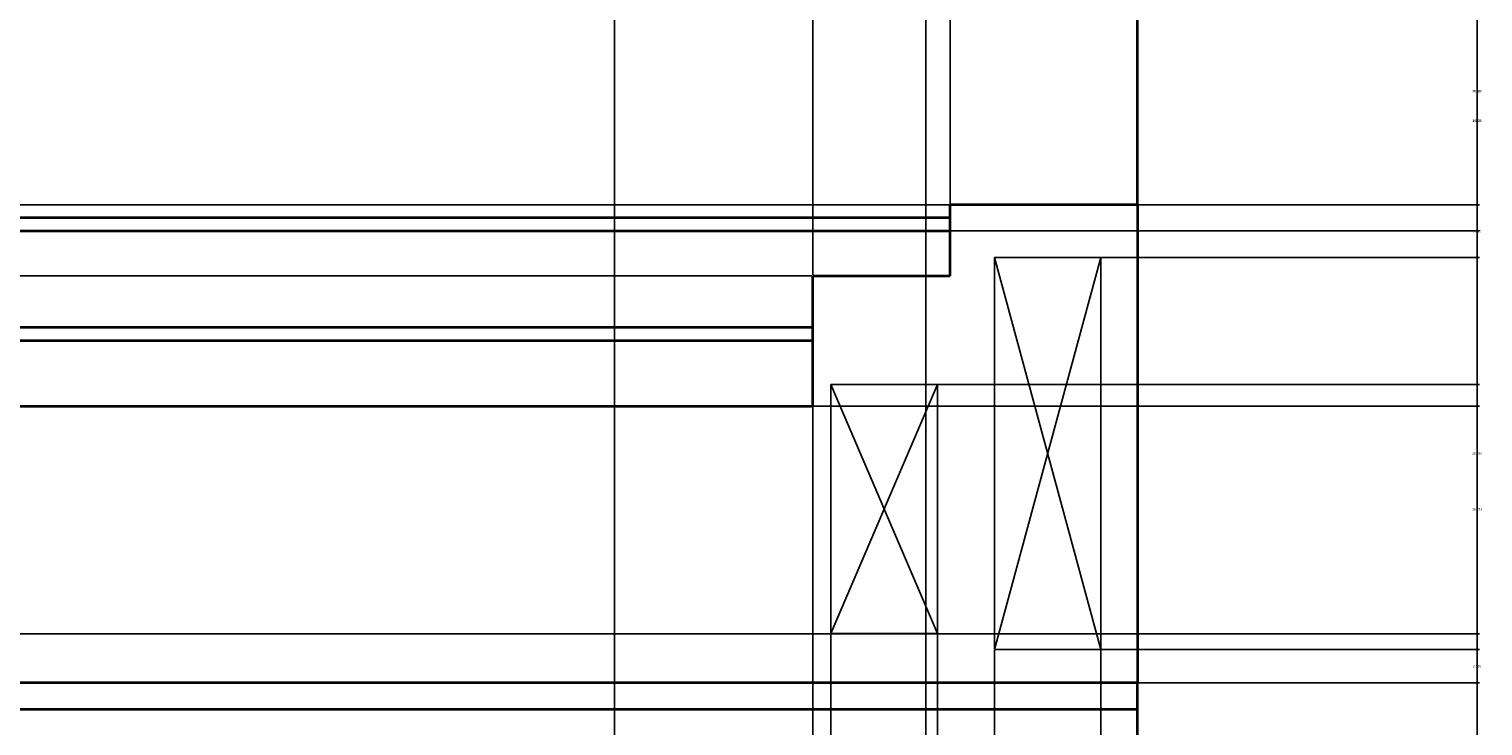
# Model space of a CAD drawing. Units: inches. Extents: x 93 to 565, y 123 to 656.
# Tile 11 of 18: x 456 to 565, y 324 to 377. Entities that reach past the tile are written whole.
import ezdxf

# ---------------------------------------------------------------- set-up
doc = ezdxf.new("R2010")
doc.units = ezdxf.units.IN
doc.header["$MEASUREMENT"] = 0
for name, color, linetype, lineweight in [('A-ANNO-DIMS', 2, 'Continuous', 18), ('A-ELEV', 7, 'Continuous', 35), ('A-GLAZ', 4, 'Continuous', 25)]:
    doc.layers.add(name, color=color, linetype=linetype, lineweight=lineweight)
doc.styles.get("Standard").update_dxf_attribs({"font": 'arial.ttf'})
doc.dimstyles.get("Standard").update_dxf_attribs({"dimtxt": 0.18, "dimasz": 0.18, "dimexe": 0.18, "dimexo": 0.0625, "dimgap": 0.09, "dimtad": 0, "dimtih": 1, "dimtoh": 1, "dimdec": 4, "dimzin": 0, "dimdsep": 46, "dimtxsty": 'Standard', "dimcen": 0.09, "dimadec": 0, "dimazin": 0, "dimtfac": 1, "dimtdec": 4, "dimtofl": 0, "dimtmove": 0, "dimatfit": 3, "dimfxl": 1, "dimtolj": 1, "dimtzin": 0, "dimarcsym": 0})

# ---------------------------------------------------------------- blocks, each defined once
blk = doc.blocks.new('*U8')
for p, q in [((0, 0), (38, 140)), ((38, 0), (0, 140))]:
    blk.add_line(p, q)
blk.add_lwpolyline([(0, 0), (38, 0), (38, 140), (0, 140)], close=True)
blk = doc.blocks.new('*U9')
for p, q in [((0, 0), (38, 89)), ((38, 0), (0, 89))]:
    blk.add_line(p, q)
blk.add_lwpolyline([(0, 0), (38, 0), (38, 89), (0, 89)], close=True)
blk = doc.blocks.new('*D30')
at = {"layer": 'A-ANNO-DIMS', "color": 0, "lineweight": -2, "transparency": 16777216}
for p, q in [((437.19, 594.34), (437.19, 134)), ((539.08, 159.67), (539.08, 134)), ((437.37, 134.18), (487.75, 134.18)), ((538.9, 134.18), (488.52, 134.18))]:
    blk.add_line(p, q, dxfattribs=at)
at = {"layer": 'A-ANNO-DIMS', "color": 0, "transparency": 16777216}
for points in [[(437.37, 134.21), (437.37, 134.15), (437.19, 134.18)], [(538.9, 134.21), (538.9, 134.15), (539.08, 134.18)]]:
    blk.add_solid(points, dxfattribs=at)
at = {"layer": 'Defpoints', "color": 0, "transparency": 16777216}
for p in [(437.19, 594.4), (539.08, 159.73), (539.08, 134.18)]:
    blk.add_point(p, dxfattribs=at)
at = {"layer": 'A-ANNO-DIMS', "color": 0, "transparency": 16777216, "insert": (488.13, 134.18), "char_height": 0.18, "attachment_point": 5}
blk.add_mtext('\\A1;101.9', dxfattribs=at)
blk = doc.blocks.new('*D31')
at = {"layer": 'A-ANNO-DIMS', "color": 0, "lineweight": -2, "transparency": 16777216}
for p, q in [((417.87, 630.4), (564.81, 630.4)), ((564.63, 630.22), (564.63, 395.25)), ((564.63, 159.91), (564.63, 394.89)), ((119.14, 159.73), (564.81, 159.73))]:
    blk.add_line(p, q, dxfattribs=at)
at = {"layer": 'A-ANNO-DIMS', "color": 0, "transparency": 16777216}
for points in [[(564.6, 630.22), (564.66, 630.22), (564.63, 630.4)], [(564.6, 159.91), (564.66, 159.91), (564.63, 159.73)]]:
    blk.add_solid(points, dxfattribs=at)
at = {"layer": 'Defpoints', "color": 0, "transparency": 16777216}
for p in [(417.81, 630.4), (564.63, 630.4), (119.08, 159.73)]:
    blk.add_point(p, dxfattribs=at)
at = {"layer": 'A-ANNO-DIMS', "color": 0, "transparency": 16777216, "insert": (564.63, 395.07), "char_height": 0.18, "attachment_point": 5}
blk.add_mtext('\\A1;470.7', dxfattribs=at)
blk = doc.blocks.new('*D37')
at = {"layer": 'A-ANNO-DIMS', "color": 0, "lineweight": -2, "transparency": 16777216}
for p, q in [((539.14, 327.73), (564.81, 327.73)), ((564.63, 327.55), (564.63, 320.52)), ((564.63, 313.13), (564.63, 320.16)), ((539.14, 312.95), (564.81, 312.95))]:
    blk.add_line(p, q, dxfattribs=at)
at = {"layer": 'A-ANNO-DIMS', "color": 0, "transparency": 16777216}
for points in [[(564.6, 327.55), (564.66, 327.55), (564.63, 327.73)], [(564.6, 313.13), (564.66, 313.13), (564.63, 312.95)]]:
    blk.add_solid(points, dxfattribs=at)
at = {"layer": 'Defpoints', "color": 0, "transparency": 16777216}
for p in [(539.08, 327.73), (564.63, 327.73), (539.08, 312.95)]:
    blk.add_point(p, dxfattribs=at)
at = {"layer": 'A-ANNO-DIMS', "color": 0, "transparency": 16777216, "insert": (564.63, 320.34), "char_height": 0.18, "attachment_point": 5}
blk.add_mtext('\\A1;14.783', dxfattribs=at)
blk = doc.blocks.new('*D67')
at = {"layer": 'A-ANNO-DIMS', "color": 0, "lineweight": -2, "transparency": 16777216}
for p, q in [((331.87, 420.57), (564.81, 420.57)), ((564.63, 420.39), (564.63, 384.75)), ((564.63, 348.75), (564.63, 384.39)), ((331.87, 348.57), (564.81, 348.57))]:
    blk.add_line(p, q, dxfattribs=at)
at = {"layer": 'A-ANNO-DIMS', "color": 0, "transparency": 16777216}
for points in [[(564.6, 420.39), (564.66, 420.39), (564.63, 420.57)], [(564.6, 348.75), (564.66, 348.75), (564.63, 348.57)]]:
    blk.add_solid(points, dxfattribs=at)
at = {"layer": 'Defpoints', "color": 0, "transparency": 16777216}
for p in [(331.81, 420.57), (564.63, 420.57), (331.81, 348.57)]:
    blk.add_point(p, dxfattribs=at)
at = {"layer": 'A-ANNO-DIMS', "color": 0, "transparency": 16777216, "insert": (564.63, 384.57), "char_height": 0.18, "attachment_point": 5}
blk.add_mtext('\\A1;72', dxfattribs=at)
blk = doc.blocks.new('*D71')
at = {"layer": 'A-ANNO-DIMS', "color": 0, "lineweight": -2, "transparency": 16777216}
for p, q in [((428.68, 382.8), (564.81, 382.8)), ((564.63, 382.62), (564.63, 372.46)), ((564.63, 361.93), (564.63, 372.09)), ((437.25, 361.75), (564.81, 361.75))]:
    blk.add_line(p, q, dxfattribs=at)
at = {"layer": 'A-ANNO-DIMS', "color": 0, "transparency": 16777216}
for points in [[(564.6, 382.62), (564.66, 382.62), (564.63, 382.8)], [(564.6, 361.93), (564.66, 361.93), (564.63, 361.75)]]:
    blk.add_solid(points, dxfattribs=at)
at = {"layer": 'Defpoints', "color": 0, "transparency": 16777216}
for p in [(428.62, 382.8), (437.19, 361.75), (564.63, 361.75)]:
    blk.add_point(p, dxfattribs=at)
at = {"layer": 'A-ANNO-DIMS', "color": 0, "transparency": 16777216, "insert": (564.63, 372.27), "char_height": 0.18, "attachment_point": 5}
blk.add_mtext('\\A1;21.05', dxfattribs=at)
blk = doc.blocks.new('*D83')
at = {"layer": 'A-ANNO-DIMS', "color": 0, "lineweight": -2, "transparency": 16777216}
for p, q in [((457.46, 378.34), (564.81, 378.34)), ((564.63, 378.16), (564.63, 370.22)), ((564.63, 361.93), (564.63, 369.86)), ((437.25, 361.75), (564.81, 361.75))]:
    blk.add_line(p, q, dxfattribs=at)
at = {"layer": 'A-ANNO-DIMS', "color": 0, "transparency": 16777216}
for points in [[(564.6, 378.16), (564.66, 378.16), (564.63, 378.34)], [(564.6, 361.93), (564.66, 361.93), (564.63, 361.75)]]:
    blk.add_solid(points, dxfattribs=at)
at = {"layer": 'Defpoints', "color": 0, "transparency": 16777216}
for p in [(457.39, 378.34), (437.19, 361.75), (564.63, 361.75)]:
    blk.add_point(p, dxfattribs=at)
at = {"layer": 'A-ANNO-DIMS', "color": 0, "transparency": 16777216, "insert": (564.63, 370.04), "char_height": 0.18, "attachment_point": 5}
blk.add_mtext('\\A1;16.59', dxfattribs=at)
blk = doc.blocks.new('*D91')
at = {"layer": 'A-ANNO-DIMS', "color": 0, "lineweight": -2, "transparency": 16777216}
for p, q in [((499.73, 599.75), (499.73, 134)), ((437.19, 594.34), (437.19, 134)), ((437.37, 134.18), (468.07, 134.18)), ((499.55, 134.18), (468.85, 134.18))]:
    blk.add_line(p, q, dxfattribs=at)
at = {"layer": 'A-ANNO-DIMS', "color": 0, "transparency": 16777216}
for points in [[(437.37, 134.21), (437.37, 134.15), (437.19, 134.18)], [(499.55, 134.21), (499.55, 134.15), (499.73, 134.18)]]:
    blk.add_solid(points, dxfattribs=at)
at = {"layer": 'Defpoints', "color": 0, "transparency": 16777216}
for p in [(499.73, 599.82), (437.19, 594.4), (499.73, 134.18)]:
    blk.add_point(p, dxfattribs=at)
at = {"layer": 'A-ANNO-DIMS', "color": 0, "transparency": 16777216, "insert": (468.46, 134.18), "char_height": 0.18, "attachment_point": 5}
blk.add_mtext('\\A1;62.54', dxfattribs=at)
blk = doc.blocks.new('*D92')
at = {"layer": 'A-ANNO-DIMS', "color": 0, "lineweight": -2, "transparency": 16777216}
for p, q in [((523.14, 603.14), (523.14, 134)), ((499.73, 599.75), (499.73, 134)), ((499.91, 134.18), (510.97, 134.18)), ((522.96, 134.18), (511.9, 134.18))]:
    blk.add_line(p, q, dxfattribs=at)
at = {"layer": 'A-ANNO-DIMS', "color": 0, "transparency": 16777216}
for points in [[(499.91, 134.21), (499.91, 134.15), (499.73, 134.18)], [(522.96, 134.21), (522.96, 134.15), (523.14, 134.18)]]:
    blk.add_solid(points, dxfattribs=at)
at = {"layer": 'Defpoints', "color": 0, "transparency": 16777216}
for p in [(523.14, 603.2), (499.73, 599.82), (523.14, 134.18)]:
    blk.add_point(p, dxfattribs=at)
at = {"layer": 'A-ANNO-DIMS', "color": 0, "transparency": 16777216, "insert": (511.44, 134.18), "char_height": 0.18, "attachment_point": 5}
blk.add_mtext('\\A1;23.412', dxfattribs=at)
blk = doc.blocks.new('*D93')
at = {"layer": 'A-ANNO-DIMS', "color": 0, "lineweight": -2, "transparency": 16777216}
for p, q in [((523.14, 603.14), (523.14, 134)), ((539.08, 594.34), (539.08, 134)), ((523.32, 134.18), (530.66, 134.18)), ((538.9, 134.18), (531.57, 134.18))]:
    blk.add_line(p, q, dxfattribs=at)
at = {"layer": 'A-ANNO-DIMS', "color": 0, "transparency": 16777216}
for points in [[(523.32, 134.21), (523.32, 134.15), (523.14, 134.18)], [(538.9, 134.21), (538.9, 134.15), (539.08, 134.18)]]:
    blk.add_solid(points, dxfattribs=at)
at = {"layer": 'Defpoints', "color": 0, "transparency": 16777216}
for p in [(523.14, 603.2), (539.08, 594.4), (539.08, 134.18)]:
    blk.add_point(p, dxfattribs=at)
at = {"layer": 'A-ANNO-DIMS', "color": 0, "transparency": 16777216, "insert": (531.11, 134.18), "char_height": 0.18, "attachment_point": 5}
blk.add_mtext('\\A1;15.938', dxfattribs=at)
blk = doc.blocks.new('*D109')
at = {"layer": 'A-ANNO-DIMS', "color": 0, "lineweight": -2, "transparency": 16777216}
for p, q in [((437.19, 594.34), (437.19, 134)), ((539.08, 159.67), (539.08, 134)), ((437.37, 134.18), (487.63, 134.18)), ((538.9, 134.18), (488.64, 134.18))]:
    blk.add_line(p, q, dxfattribs=at)
at = {"layer": 'A-ANNO-DIMS', "color": 0, "transparency": 16777216}
for points in [[(437.37, 134.21), (437.37, 134.15), (437.19, 134.18)], [(538.9, 134.21), (538.9, 134.15), (539.08, 134.18)]]:
    blk.add_solid(points, dxfattribs=at)
at = {"layer": 'Defpoints', "color": 0, "transparency": 16777216}
for p in [(437.19, 594.4), (539.08, 159.73), (539.08, 134.18)]:
    blk.add_point(p, dxfattribs=at)
at = {"layer": 'A-ANNO-DIMS', "color": 0, "transparency": 16777216, "insert": (488.13, 134.18), "char_height": 0.18, "attachment_point": 5}
blk.add_mtext('\\A1;101.891', dxfattribs=at)
blk = doc.blocks.new('*D110')
at = {"layer": 'A-ANNO-DIMS', "color": 0, "lineweight": -2, "transparency": 16777216}
for p, q in [((417.87, 630.4), (564.81, 630.4)), ((564.63, 630.22), (564.63, 395.25)), ((564.63, 159.91), (564.63, 394.89)), ((119.14, 159.73), (564.81, 159.73))]:
    blk.add_line(p, q, dxfattribs=at)
at = {"layer": 'A-ANNO-DIMS', "color": 0, "transparency": 16777216}
for points in [[(564.6, 630.22), (564.66, 630.22), (564.63, 630.4)], [(564.6, 159.91), (564.66, 159.91), (564.63, 159.73)]]:
    blk.add_solid(points, dxfattribs=at)
at = {"layer": 'Defpoints', "color": 0, "transparency": 16777216}
for p in [(417.81, 630.4), (564.63, 630.4), (119.08, 159.73)]:
    blk.add_point(p, dxfattribs=at)
at = {"layer": 'A-ANNO-DIMS', "color": 0, "transparency": 16777216, "insert": (564.63, 395.07), "char_height": 0.18, "attachment_point": 5}
blk.add_mtext('\\A1;470.673', dxfattribs=at)
blk = doc.blocks.new('*D116')
at = {"layer": 'A-ANNO-DIMS', "color": 0, "lineweight": -2, "transparency": 16777216}
for p, q in [((539.14, 327.73), (564.81, 327.73)), ((564.63, 327.55), (564.63, 320.52)), ((564.63, 313.13), (564.63, 320.16)), ((539.14, 312.95), (564.81, 312.95))]:
    blk.add_line(p, q, dxfattribs=at)
at = {"layer": 'A-ANNO-DIMS', "color": 0, "transparency": 16777216}
for points in [[(564.6, 327.55), (564.66, 327.55), (564.63, 327.73)], [(564.6, 313.13), (564.66, 313.13), (564.63, 312.95)]]:
    blk.add_solid(points, dxfattribs=at)
at = {"layer": 'Defpoints', "color": 0, "transparency": 16777216}
for p in [(539.08, 327.73), (564.63, 327.73), (539.08, 312.95)]:
    blk.add_point(p, dxfattribs=at)
at = {"layer": 'A-ANNO-DIMS', "color": 0, "transparency": 16777216, "insert": (564.63, 320.34), "char_height": 0.18, "attachment_point": 5}
blk.add_mtext('\\A1;14.783', dxfattribs=at)
blk = doc.blocks.new('*D146')
at = {"layer": 'A-ANNO-DIMS', "color": 0, "lineweight": -2, "transparency": 16777216}
for p, q in [((331.87, 420.57), (564.81, 420.57)), ((564.63, 420.39), (564.63, 384.75)), ((564.63, 348.75), (564.63, 384.39)), ((331.87, 348.57), (564.81, 348.57))]:
    blk.add_line(p, q, dxfattribs=at)
at = {"layer": 'A-ANNO-DIMS', "color": 0, "transparency": 16777216}
for points in [[(564.6, 420.39), (564.66, 420.39), (564.63, 420.57)], [(564.6, 348.75), (564.66, 348.75), (564.63, 348.57)]]:
    blk.add_solid(points, dxfattribs=at)
at = {"layer": 'Defpoints', "color": 0, "transparency": 16777216}
for p in [(331.81, 420.57), (564.63, 420.57), (331.81, 348.57)]:
    blk.add_point(p, dxfattribs=at)
at = {"layer": 'A-ANNO-DIMS', "color": 0, "transparency": 16777216, "insert": (564.63, 384.57), "char_height": 0.18, "attachment_point": 5}
blk.add_mtext('\\A1;72.000', dxfattribs=at)
blk = doc.blocks.new('*D150')
at = {"layer": 'A-ANNO-DIMS', "color": 0, "lineweight": -2, "transparency": 16777216}
for p, q in [((428.68, 382.8), (564.81, 382.8)), ((564.63, 382.62), (564.63, 372.46)), ((564.63, 361.93), (564.63, 372.09)), ((437.25, 361.75), (564.81, 361.75))]:
    blk.add_line(p, q, dxfattribs=at)
at = {"layer": 'A-ANNO-DIMS', "color": 0, "transparency": 16777216}
for points in [[(564.6, 382.62), (564.66, 382.62), (564.63, 382.8)], [(564.6, 361.93), (564.66, 361.93), (564.63, 361.75)]]:
    blk.add_solid(points, dxfattribs=at)
at = {"layer": 'Defpoints', "color": 0, "transparency": 16777216}
for p in [(428.62, 382.8), (437.19, 361.75), (564.63, 361.75)]:
    blk.add_point(p, dxfattribs=at)
at = {"layer": 'A-ANNO-DIMS', "color": 0, "transparency": 16777216, "insert": (564.63, 372.27), "char_height": 0.18, "attachment_point": 5}
blk.add_mtext('\\A1;21.052', dxfattribs=at)
blk = doc.blocks.new('*D162')
at = {"layer": 'A-ANNO-DIMS', "color": 0, "lineweight": -2, "transparency": 16777216}
for p, q in [((457.46, 378.34), (564.81, 378.34)), ((564.63, 378.16), (564.63, 370.22)), ((564.63, 361.93), (564.63, 369.86)), ((437.25, 361.75), (564.81, 361.75))]:
    blk.add_line(p, q, dxfattribs=at)
at = {"layer": 'A-ANNO-DIMS', "color": 0, "transparency": 16777216}
for points in [[(564.6, 378.16), (564.66, 378.16), (564.63, 378.34)], [(564.6, 361.93), (564.66, 361.93), (564.63, 361.75)]]:
    blk.add_solid(points, dxfattribs=at)
at = {"layer": 'Defpoints', "color": 0, "transparency": 16777216}
for p in [(457.39, 378.34), (437.19, 361.75), (564.63, 361.75)]:
    blk.add_point(p, dxfattribs=at)
at = {"layer": 'A-ANNO-DIMS', "color": 0, "transparency": 16777216, "insert": (564.63, 370.04), "char_height": 0.18, "attachment_point": 5}
blk.add_mtext('\\A1;16.590', dxfattribs=at)
blk = doc.blocks.new('*D170')
at = {"layer": 'A-ANNO-DIMS', "color": 0, "lineweight": -2, "transparency": 16777216}
for p, q in [((499.73, 599.75), (499.73, 134)), ((437.19, 594.34), (437.19, 134)), ((437.37, 134.18), (468.01, 134.18)), ((499.55, 134.18), (468.91, 134.18))]:
    blk.add_line(p, q, dxfattribs=at)
at = {"layer": 'A-ANNO-DIMS', "color": 0, "transparency": 16777216}
for points in [[(437.37, 134.21), (437.37, 134.15), (437.19, 134.18)], [(499.55, 134.21), (499.55, 134.15), (499.73, 134.18)]]:
    blk.add_solid(points, dxfattribs=at)
at = {"layer": 'Defpoints', "color": 0, "transparency": 16777216}
for p in [(499.73, 599.82), (437.19, 594.4), (499.73, 134.18)]:
    blk.add_point(p, dxfattribs=at)
at = {"layer": 'A-ANNO-DIMS', "color": 0, "transparency": 16777216, "insert": (468.46, 134.18), "char_height": 0.18, "attachment_point": 5}
blk.add_mtext('\\A1;62.541', dxfattribs=at)
blk = doc.blocks.new('*D171')
at = {"layer": 'A-ANNO-DIMS', "color": 0, "lineweight": -2, "transparency": 16777216}
for p, q in [((523.14, 603.14), (523.14, 134)), ((499.73, 599.75), (499.73, 134)), ((499.91, 134.18), (510.97, 134.18)), ((522.96, 134.18), (511.9, 134.18))]:
    blk.add_line(p, q, dxfattribs=at)
at = {"layer": 'A-ANNO-DIMS', "color": 0, "transparency": 16777216}
for points in [[(499.91, 134.21), (499.91, 134.15), (499.73, 134.18)], [(522.96, 134.21), (522.96, 134.15), (523.14, 134.18)]]:
    blk.add_solid(points, dxfattribs=at)
at = {"layer": 'Defpoints', "color": 0, "transparency": 16777216}
for p in [(523.14, 603.2), (499.73, 599.82), (523.14, 134.18)]:
    blk.add_point(p, dxfattribs=at)
at = {"layer": 'A-ANNO-DIMS', "color": 0, "transparency": 16777216, "insert": (511.44, 134.18), "char_height": 0.18, "attachment_point": 5}
blk.add_mtext('\\A1;23.412', dxfattribs=at)
blk = doc.blocks.new('*D172')
at = {"layer": 'A-ANNO-DIMS', "color": 0, "lineweight": -2, "transparency": 16777216}
for p, q in [((523.14, 603.14), (523.14, 134)), ((539.08, 594.34), (539.08, 134)), ((523.32, 134.18), (530.66, 134.18)), ((538.9, 134.18), (531.57, 134.18))]:
    blk.add_line(p, q, dxfattribs=at)
at = {"layer": 'A-ANNO-DIMS', "color": 0, "transparency": 16777216}
for points in [[(523.32, 134.21), (523.32, 134.15), (523.14, 134.18)], [(538.9, 134.21), (538.9, 134.15), (539.08, 134.18)]]:
    blk.add_solid(points, dxfattribs=at)
at = {"layer": 'Defpoints', "color": 0, "transparency": 16777216}
for p in [(523.14, 603.2), (539.08, 594.4), (539.08, 134.18)]:
    blk.add_point(p, dxfattribs=at)
at = {"layer": 'A-ANNO-DIMS', "color": 0, "transparency": 16777216, "insert": (531.11, 134.18), "char_height": 0.18, "attachment_point": 5}
blk.add_mtext('\\A1;15.938', dxfattribs=at)
blk = doc.blocks.new('*D180')
at = {"layer": 'A-ANNO-DIMS', "color": 0, "lineweight": -2, "transparency": 16777216}
for p, q in [((514.64, 348.49), (514.64, 134)), ((516.01, 331.37), (516.01, 134)), ((514.82, 134.18), (514.94, 134.18)), ((515.83, 134.18), (515.71, 134.18))]:
    blk.add_line(p, q, dxfattribs=at)
at = {"layer": 'A-ANNO-DIMS', "color": 0, "transparency": 16777216}
for points in [[(514.82, 134.21), (514.82, 134.15), (514.64, 134.18)], [(515.83, 134.21), (515.83, 134.15), (516.01, 134.18)]]:
    blk.add_solid(points, dxfattribs=at)
at = {"layer": 'Defpoints', "color": 0, "transparency": 16777216}
for p in [(514.64, 348.55), (516.01, 331.43), (516.01, 134.18)]:
    blk.add_point(p, dxfattribs=at)
at = {"layer": 'A-ANNO-DIMS', "color": 0, "transparency": 16777216, "insert": (515.33, 134.18), "char_height": 0.18, "attachment_point": 5}
blk.add_mtext('\\A1;1.367', dxfattribs=at)
blk = doc.blocks.new('*D181')
at = {"layer": 'A-ANNO-DIMS', "color": 0, "lineweight": -2, "transparency": 16777216}
for p, q in [((516.01, 331.37), (516.01, 134)), ((524.02, 331.37), (524.02, 134)), ((516.19, 134.18), (519.62, 134.18)), ((523.84, 134.18), (520.41, 134.18))]:
    blk.add_line(p, q, dxfattribs=at)
at = {"layer": 'A-ANNO-DIMS', "color": 0, "transparency": 16777216}
for points in [[(516.19, 134.21), (516.19, 134.15), (516.01, 134.18)], [(523.84, 134.21), (523.84, 134.15), (524.02, 134.18)]]:
    blk.add_solid(points, dxfattribs=at)
at = {"layer": 'Defpoints', "color": 0, "transparency": 16777216}
for p in [(516.01, 331.43), (524.02, 331.43), (524.02, 134.18)]:
    blk.add_point(p, dxfattribs=at)
at = {"layer": 'A-ANNO-DIMS', "color": 0, "transparency": 16777216, "insert": (520.01, 134.18), "char_height": 0.18, "attachment_point": 5}
blk.add_mtext('\\A1;8.007', dxfattribs=at)
blk = doc.blocks.new('*D182')
at = {"layer": 'A-ANNO-DIMS', "color": 0, "lineweight": -2, "transparency": 16777216}
for p, q in [((524.02, 331.37), (524.02, 134)), ((528.31, 330.19), (528.31, 134)), ((524.2, 134.18), (525.77, 134.18)), ((528.13, 134.18), (526.56, 134.18))]:
    blk.add_line(p, q, dxfattribs=at)
at = {"layer": 'A-ANNO-DIMS', "color": 0, "transparency": 16777216}
for points in [[(524.2, 134.21), (524.2, 134.15), (524.02, 134.18)], [(528.13, 134.21), (528.13, 134.15), (528.31, 134.18)]]:
    blk.add_solid(points, dxfattribs=at)
at = {"layer": 'Defpoints', "color": 0, "transparency": 16777216}
for p in [(524.02, 331.43), (528.31, 330.25), (528.31, 134.18)]:
    blk.add_point(p, dxfattribs=at)
at = {"layer": 'A-ANNO-DIMS', "color": 0, "transparency": 16777216, "insert": (526.17, 134.18), "char_height": 0.18, "attachment_point": 5}
blk.add_mtext('\\A1;4.297', dxfattribs=at)
blk = doc.blocks.new('*D183')
at = {"layer": 'A-ANNO-DIMS', "color": 0, "lineweight": -2, "transparency": 16777216}
for p, q in [((528.31, 330.19), (528.31, 134)), ((536.32, 330.19), (536.32, 134)), ((528.49, 134.18), (531.92, 134.18)), ((536.14, 134.18), (532.71, 134.18))]:
    blk.add_line(p, q, dxfattribs=at)
at = {"layer": 'A-ANNO-DIMS', "color": 0, "transparency": 16777216}
for points in [[(528.49, 134.21), (528.49, 134.15), (528.31, 134.18)], [(536.14, 134.21), (536.14, 134.15), (536.32, 134.18)]]:
    blk.add_solid(points, dxfattribs=at)
at = {"layer": 'Defpoints', "color": 0, "transparency": 16777216}
for p in [(528.31, 330.25), (536.32, 330.25), (536.32, 134.18)]:
    blk.add_point(p, dxfattribs=at)
at = {"layer": 'A-ANNO-DIMS', "color": 0, "transparency": 16777216, "insert": (532.32, 134.18), "char_height": 0.18, "attachment_point": 5}
blk.add_mtext('\\A1;8.007', dxfattribs=at)
blk = doc.blocks.new('*D184')
at = {"layer": 'A-ANNO-DIMS', "color": 0, "lineweight": -2, "transparency": 16777216}
for p, q in [((536.32, 330.19), (536.32, 134)), ((539.08, 327.67), (539.08, 134)), ((536.5, 134.18), (537.31, 134.18)), ((538.9, 134.18), (538.1, 134.18))]:
    blk.add_line(p, q, dxfattribs=at)
at = {"layer": 'A-ANNO-DIMS', "color": 0, "transparency": 16777216}
for points in [[(536.5, 134.21), (536.5, 134.15), (536.32, 134.18)], [(538.9, 134.21), (538.9, 134.15), (539.08, 134.18)]]:
    blk.add_solid(points, dxfattribs=at)
at = {"layer": 'Defpoints', "color": 0, "transparency": 16777216}
for p in [(536.32, 330.25), (539.08, 327.73), (539.08, 134.18)]:
    blk.add_point(p, dxfattribs=at)
at = {"layer": 'A-ANNO-DIMS', "color": 0, "transparency": 16777216, "insert": (537.7, 134.18), "char_height": 0.18, "attachment_point": 5}
blk.add_mtext('\\A1;2.758', dxfattribs=at)
blk = doc.blocks.new('*D185')
at = {"layer": 'A-ANNO-DIMS', "color": 0, "lineweight": -2, "transparency": 16777216}
for p, q in [((514.64, 358.44), (514.64, 656.13)), ((514.82, 655.95), (519.36, 655.95)), ((524.81, 655.95), (520.27, 655.95)), ((524.99, 363.79), (524.99, 656.13))]:
    blk.add_line(p, q, dxfattribs=at)
at = {"layer": 'A-ANNO-DIMS', "color": 0, "transparency": 16777216}
for points in [[(514.82, 655.98), (514.82, 655.92), (514.64, 655.95)], [(524.81, 655.98), (524.81, 655.92), (524.99, 655.95)]]:
    blk.add_solid(points, dxfattribs=at)
at = {"layer": 'Defpoints', "color": 0, "transparency": 16777216}
for p in [(524.99, 655.95), (524.99, 363.73), (514.64, 358.37)]:
    blk.add_point(p, dxfattribs=at)
at = {"layer": 'A-ANNO-DIMS', "color": 0, "transparency": 16777216, "insert": (519.81, 655.95), "char_height": 0.18, "attachment_point": 5}
blk.add_mtext('\\A1;10.344', dxfattribs=at)
blk = doc.blocks.new('*D186')
at = {"layer": 'A-ANNO-DIMS', "color": 0, "lineweight": -2, "transparency": 16777216}
for p, q in [((524.99, 363.79), (524.99, 656.13)), ((525.17, 655.95), (531.58, 655.95)), ((538.9, 655.95), (532.49, 655.95)), ((539.08, 363.79), (539.08, 656.13))]:
    blk.add_line(p, q, dxfattribs=at)
at = {"layer": 'A-ANNO-DIMS', "color": 0, "transparency": 16777216}
for points in [[(525.17, 655.98), (525.17, 655.92), (524.99, 655.95)], [(538.9, 655.98), (538.9, 655.92), (539.08, 655.95)]]:
    blk.add_solid(points, dxfattribs=at)
at = {"layer": 'Defpoints', "color": 0, "transparency": 16777216}
for p in [(539.08, 655.95), (524.99, 363.73), (539.08, 363.73)]:
    blk.add_point(p, dxfattribs=at)
at = {"layer": 'A-ANNO-DIMS', "color": 0, "transparency": 16777216, "insert": (532.03, 655.95), "char_height": 0.18, "attachment_point": 5}
blk.add_mtext('\\A1;14.093', dxfattribs=at)
blk = doc.blocks.new('*D187')
at = {"layer": 'A-ANNO-DIMS', "color": 0, "lineweight": -2, "transparency": 16777216}
for p, q in [((536.38, 330.25), (564.81, 330.25)), ((564.63, 330.07), (564.63, 329.17)), ((564.63, 327.91), (564.63, 328.81)), ((539.14, 327.73), (564.81, 327.73))]:
    blk.add_line(p, q, dxfattribs=at)
at = {"layer": 'A-ANNO-DIMS', "color": 0, "transparency": 16777216}
for points in [[(564.6, 330.07), (564.66, 330.07), (564.63, 330.25)], [(564.6, 327.91), (564.66, 327.91), (564.63, 327.73)]]:
    blk.add_solid(points, dxfattribs=at)
at = {"layer": 'Defpoints', "color": 0, "transparency": 16777216}
for p in [(536.32, 330.25), (564.63, 330.25), (539.08, 327.73)]:
    blk.add_point(p, dxfattribs=at)
at = {"layer": 'A-ANNO-DIMS', "color": 0, "transparency": 16777216, "insert": (564.63, 328.99), "char_height": 0.18, "attachment_point": 5}
blk.add_mtext('\\A1;2.516', dxfattribs=at)
blk = doc.blocks.new('*D188')
at = {"layer": 'A-ANNO-DIMS', "color": 0, "lineweight": -2, "transparency": 16777216}
for p, q in [((536.38, 359.75), (564.81, 359.75)), ((564.63, 359.57), (564.63, 345.18)), ((564.63, 330.43), (564.63, 344.82)), ((536.38, 330.25), (564.81, 330.25))]:
    blk.add_line(p, q, dxfattribs=at)
at = {"layer": 'A-ANNO-DIMS', "color": 0, "transparency": 16777216}
for points in [[(564.6, 359.57), (564.66, 359.57), (564.63, 359.75)], [(564.6, 330.43), (564.66, 330.43), (564.63, 330.25)]]:
    blk.add_solid(points, dxfattribs=at)
at = {"layer": 'Defpoints', "color": 0, "transparency": 16777216}
for p in [(536.32, 359.75), (564.63, 359.75), (536.32, 330.25)]:
    blk.add_point(p, dxfattribs=at)
at = {"layer": 'A-ANNO-DIMS', "color": 0, "transparency": 16777216, "insert": (564.63, 345), "char_height": 0.18, "attachment_point": 5}
blk.add_mtext('\\A1;29.500', dxfattribs=at)
blk = doc.blocks.new('*D189')
at = {"layer": 'A-ANNO-DIMS', "color": 0, "lineweight": -2, "transparency": 16777216}
for p, q in [((539.14, 363.73), (564.81, 363.73)), ((564.63, 363.55), (564.63, 361.92)), ((564.63, 359.93), (564.63, 361.56)), ((536.38, 359.75), (564.81, 359.75))]:
    blk.add_line(p, q, dxfattribs=at)
at = {"layer": 'A-ANNO-DIMS', "color": 0, "transparency": 16777216}
for points in [[(564.6, 363.55), (564.66, 363.55), (564.63, 363.73)], [(564.6, 359.93), (564.66, 359.93), (564.63, 359.75)]]:
    blk.add_solid(points, dxfattribs=at)
at = {"layer": 'Defpoints', "color": 0, "transparency": 16777216}
for p in [(539.08, 363.73), (564.63, 363.73), (536.32, 359.75)]:
    blk.add_point(p, dxfattribs=at)
at = {"layer": 'A-ANNO-DIMS', "color": 0, "transparency": 16777216, "insert": (564.63, 361.74), "char_height": 0.18, "attachment_point": 5}
blk.add_mtext('\\A1;3.985', dxfattribs=at)
blk = doc.blocks.new('*D190')
at = {"layer": 'A-ANNO-DIMS', "color": 0, "lineweight": -2, "transparency": 16777216}
for p, q in [((514.58, 348.55), (93.35, 348.55)), ((93.53, 348.37), (93.53, 338.33)), ((93.53, 327.91), (93.53, 337.96)), ((539.02, 327.73), (93.35, 327.73))]:
    blk.add_line(p, q, dxfattribs=at)
at = {"layer": 'A-ANNO-DIMS', "color": 0, "transparency": 16777216}
for points in [[(93.5, 348.37), (93.56, 348.37), (93.53, 348.55)], [(93.5, 327.91), (93.56, 327.91), (93.53, 327.73)]]:
    blk.add_solid(points, dxfattribs=at)
at = {"layer": 'Defpoints', "color": 0, "transparency": 16777216}
for p in [(93.53, 348.55), (514.64, 348.55), (539.08, 327.73)]:
    blk.add_point(p, dxfattribs=at)
at = {"layer": 'A-ANNO-DIMS', "color": 0, "transparency": 16777216, "insert": (93.53, 338.14), "char_height": 0.18, "attachment_point": 5}
blk.add_mtext('\\A1;20.822', dxfattribs=at)
blk = doc.blocks.new('*D191')
at = {"layer": 'A-ANNO-DIMS', "color": 0, "lineweight": -2, "transparency": 16777216}
for p, q in [((514.58, 353.47), (93.35, 353.47)), ((93.53, 353.29), (93.53, 351.2)), ((93.53, 348.73), (93.53, 350.83)), ((514.58, 348.55), (93.35, 348.55))]:
    blk.add_line(p, q, dxfattribs=at)
at = {"layer": 'A-ANNO-DIMS', "color": 0, "transparency": 16777216}
for points in [[(93.5, 353.29), (93.56, 353.29), (93.53, 353.47)], [(93.5, 348.73), (93.56, 348.73), (93.53, 348.55)]]:
    blk.add_solid(points, dxfattribs=at)
at = {"layer": 'Defpoints', "color": 0, "transparency": 16777216}
for p in [(93.53, 353.47), (514.64, 353.47), (514.64, 348.55)]:
    blk.add_point(p, dxfattribs=at)
at = {"layer": 'A-ANNO-DIMS', "color": 0, "transparency": 16777216, "insert": (93.53, 351.01), "char_height": 0.18, "attachment_point": 5}
blk.add_mtext('\\A1;4.918', dxfattribs=at)
blk = doc.blocks.new('*D192')
at = {"layer": 'A-ANNO-DIMS', "color": 0, "lineweight": -2, "transparency": 16777216}
for p, q in [((514.58, 354.47), (93.35, 354.47)), ((514.58, 353.47), (93.35, 353.47)), ((93.53, 354.29), (93.53, 354.15)), ((93.53, 353.65), (93.53, 353.79))]:
    blk.add_line(p, q, dxfattribs=at)
at = {"layer": 'A-ANNO-DIMS', "color": 0, "transparency": 16777216}
for points in [[(93.5, 354.29), (93.56, 354.29), (93.53, 354.47)], [(93.5, 353.65), (93.56, 353.65), (93.53, 353.47)]]:
    blk.add_solid(points, dxfattribs=at)
at = {"layer": 'Defpoints', "color": 0, "transparency": 16777216}
for p in [(93.53, 354.47), (514.64, 354.47), (514.64, 353.47)]:
    blk.add_point(p, dxfattribs=at)
at = {"layer": 'A-ANNO-DIMS', "color": 0, "transparency": 16777216, "insert": (93.53, 353.97), "char_height": 0.18, "attachment_point": 5}
blk.add_mtext('\\A1;1.000', dxfattribs=at)
blk = doc.blocks.new('*D193')
at = {"layer": 'A-ANNO-DIMS', "color": 0, "lineweight": -2, "transparency": 16777216}
for p, q in [((514.58, 358.37), (93.35, 358.37)), ((93.53, 358.19), (93.53, 356.61)), ((93.53, 354.65), (93.53, 356.24)), ((514.58, 354.47), (93.35, 354.47))]:
    blk.add_line(p, q, dxfattribs=at)
at = {"layer": 'A-ANNO-DIMS', "color": 0, "transparency": 16777216}
for points in [[(93.5, 358.19), (93.56, 358.19), (93.53, 358.37)], [(93.5, 354.65), (93.56, 354.65), (93.53, 354.47)]]:
    blk.add_solid(points, dxfattribs=at)
at = {"layer": 'Defpoints', "color": 0, "transparency": 16777216}
for p in [(93.53, 358.37), (514.64, 358.37), (514.64, 354.47)]:
    blk.add_point(p, dxfattribs=at)
at = {"layer": 'A-ANNO-DIMS', "color": 0, "transparency": 16777216, "insert": (93.53, 356.42), "char_height": 0.18, "attachment_point": 5}
blk.add_mtext('\\A1;3.901', dxfattribs=at)
blk = doc.blocks.new('*D194')
at = {"layer": 'A-ANNO-DIMS', "color": 0, "lineweight": -2, "transparency": 16777216}
for p, q in [((524.92, 361.75), (93.35, 361.75)), ((93.53, 361.57), (93.53, 360.24)), ((93.53, 358.55), (93.53, 359.88)), ((514.58, 358.37), (93.35, 358.37))]:
    blk.add_line(p, q, dxfattribs=at)
at = {"layer": 'A-ANNO-DIMS', "color": 0, "transparency": 16777216}
for points in [[(93.5, 361.57), (93.56, 361.57), (93.53, 361.75)], [(93.5, 358.55), (93.56, 358.55), (93.53, 358.37)]]:
    blk.add_solid(points, dxfattribs=at)
at = {"layer": 'Defpoints', "color": 0, "transparency": 16777216}
for p in [(93.53, 361.75), (524.99, 361.75), (514.64, 358.37)]:
    blk.add_point(p, dxfattribs=at)
at = {"layer": 'A-ANNO-DIMS', "color": 0, "transparency": 16777216, "insert": (93.53, 360.06), "char_height": 0.18, "attachment_point": 5}
blk.add_mtext('\\A1;3.374', dxfattribs=at)
blk = doc.blocks.new('*D195')
at = {"layer": 'A-ANNO-DIMS', "color": 0, "lineweight": -2, "transparency": 16777216}
for p, q in [((524.92, 362.75), (93.35, 362.75)), ((93.53, 362.57), (93.53, 362.43)), ((524.92, 361.75), (93.35, 361.75)), ((93.53, 361.93), (93.53, 362.07))]:
    blk.add_line(p, q, dxfattribs=at)
at = {"layer": 'A-ANNO-DIMS', "color": 0, "transparency": 16777216}
for points in [[(93.5, 362.57), (93.56, 362.57), (93.53, 362.75)], [(93.5, 361.93), (93.56, 361.93), (93.53, 361.75)]]:
    blk.add_solid(points, dxfattribs=at)
at = {"layer": 'Defpoints', "color": 0, "transparency": 16777216}
for p in [(93.53, 362.75), (524.99, 362.75), (524.99, 361.75)]:
    blk.add_point(p, dxfattribs=at)
at = {"layer": 'A-ANNO-DIMS', "color": 0, "transparency": 16777216, "insert": (93.53, 362.25), "char_height": 0.18, "attachment_point": 5}
blk.add_mtext('\\A1;1.000', dxfattribs=at)
blk = doc.blocks.new('*D196')
at = {"layer": 'A-ANNO-DIMS', "color": 0, "lineweight": -2, "transparency": 16777216}
for p, q in [((524.92, 363.73), (93.35, 363.73)), ((93.53, 363.55), (93.53, 363.42)), ((524.92, 362.75), (93.35, 362.75)), ((93.53, 362.93), (93.53, 363.06))]:
    blk.add_line(p, q, dxfattribs=at)
at = {"layer": 'A-ANNO-DIMS', "color": 0, "transparency": 16777216}
for points in [[(93.5, 363.55), (93.56, 363.55), (93.53, 363.73)], [(93.5, 362.93), (93.56, 362.93), (93.53, 362.75)]]:
    blk.add_solid(points, dxfattribs=at)
at = {"layer": 'Defpoints', "color": 0, "transparency": 16777216}
for p in [(93.53, 363.73), (524.99, 363.73), (524.99, 362.75)]:
    blk.add_point(p, dxfattribs=at)
at = {"layer": 'A-ANNO-DIMS', "color": 0, "transparency": 16777216, "insert": (93.53, 363.24), "char_height": 0.18, "attachment_point": 5}
blk.add_mtext('\\A1;0.985', dxfattribs=at)
blk = doc.blocks.new('*D197')
at = {"layer": 'A-ANNO-DIMS', "color": 0, "lineweight": -2, "transparency": 16777216}
for p, q in [((516.07, 350.19), (564.81, 350.19)), ((564.63, 350.01), (564.63, 340.99)), ((564.63, 331.61), (564.63, 340.63)), ((516.07, 331.43), (564.81, 331.43))]:
    blk.add_line(p, q, dxfattribs=at)
at = {"layer": 'A-ANNO-DIMS', "color": 0, "transparency": 16777216}
for points in [[(564.6, 350.01), (564.66, 350.01), (564.63, 350.19)], [(564.6, 331.61), (564.66, 331.61), (564.63, 331.43)]]:
    blk.add_solid(points, dxfattribs=at)
at = {"layer": 'Defpoints', "color": 0, "transparency": 16777216}
for p in [(516.01, 350.19), (564.63, 350.19), (516.01, 331.43)]:
    blk.add_point(p, dxfattribs=at)
at = {"layer": 'A-ANNO-DIMS', "color": 0, "transparency": 16777216, "insert": (564.63, 340.81), "char_height": 0.18, "attachment_point": 5}
blk.add_mtext('\\A1;18.753', dxfattribs=at)
blk = doc.blocks.new('*D198')
at = {"layer": 'A-ANNO-DIMS', "color": 0, "lineweight": -2, "transparency": 16777216}
for p, q in [((515.95, 331.43), (93.35, 331.43)), ((93.53, 331.25), (93.53, 329.76)), ((93.53, 327.91), (93.53, 329.4)), ((539.02, 327.73), (93.35, 327.73))]:
    blk.add_line(p, q, dxfattribs=at)
at = {"layer": 'A-ANNO-DIMS', "color": 0, "transparency": 16777216}
for points in [[(93.5, 331.25), (93.56, 331.25), (93.53, 331.43)], [(93.5, 327.91), (93.56, 327.91), (93.53, 327.73)]]:
    blk.add_solid(points, dxfattribs=at)
at = {"layer": 'Defpoints', "color": 0, "transparency": 16777216}
for p in [(93.53, 331.43), (516.01, 331.43), (539.08, 327.73)]:
    blk.add_point(p, dxfattribs=at)
at = {"layer": 'A-ANNO-DIMS', "color": 0, "transparency": 16777216, "insert": (93.53, 329.58), "char_height": 0.18, "attachment_point": 5}
blk.add_mtext('\\A1;3.701', dxfattribs=at)

msp = doc.modelspace()

# ---------------------------------------------------------------- linework, layer by layer
at = {"layer": 'A-ELEV'}
for p, q in [((539.0794, 363.7323), (539.0794, 594.4048)), ((524.9864, 358.3735), (524.9864, 363.7323)), ((524.9864, 363.7323), (539.0794, 363.7323)), ((539.0794, 363.7323), (539.0794, 327.7323)), ((524.9864, 362.7477), (295.6874, 362.7477)), ((524.9864, 361.7477), (295.6874, 361.7477)), ((514.6424, 348.5546), (514.6424, 358.3735)), ((514.6424, 358.3735), (524.9864, 358.3735)), ((514.6424, 354.4729), (295.6874, 354.4729)), ((514.6424, 353.4729), (295.6874, 353.4729)), ((295.6874, 348.5546), (514.6424, 348.5546)), ((539.0794, 327.7323), (295.6874, 327.7323)), ((539.0794, 183.7323), (539.0794, 327.7323)), ((539.0794, 325.7323), (295.6874, 325.7323))]:
    msp.add_line(p, q, dxfattribs=at)

# ---------------------------------------------------------------- block references
at = {"layer": 'A-GLAZ', "xscale": 0.2107133031769033, "yscale": 0.2107133031769033, "zscale": 0.2107133031769033}
for name, p in [('*U8', (528.3144, 330.2478)), ('*U9', (516.0099, 331.4335))]:
    msp.add_blockref(name, p, dxfattribs=at)

# ---------------------------------------------------------------- dimensions: what is measured, and where the dimension line sits
at = {"layer": 'A-ANNO-DIMS'}
for base, p1, p2, override, picture, middle in [((524.9864, 655.9548), (514.6424, 358.3735), (524.9864, 363.7323), {"dimdec": 3, "dimlfac": 1, "dimrnd": 0, "dimzin": 0, "dimdsep": 46, "dimlunit": 2}, '*D185', (519.8144, 655.9548)), ((539.0794, 655.9548), (524.9864, 363.7323), (539.0794, 363.7323), {"dimdec": 3, "dimlfac": 1, "dimrnd": 0, "dimzin": 0, "dimdsep": 46, "dimlunit": 2}, '*D186', (532.0329, 655.9548)), ((523.1415, 134.1823), (499.7291, 599.8171), (523.1415, 603.1979), {"dimdec": 3, "dimlfac": 1, "dimrnd": 0, "dimzin": 0, "dimdsep": 46, "dimlunit": 2}, '*D92', (511.4353, 134.1823)), ((523.1415, 134.1823), (499.7291, 599.8171), (523.1415, 603.1979), {"dimdec": 3, "dimlfac": 1, "dimrnd": 0, "dimzin": 0, "dimdsep": 46, "dimlunit": 2}, '*D171', (511.4353, 134.1823)), ((539.0794, 134.1823), (523.1415, 603.1979), (539.0794, 594.4048), {"dimdec": 3, "dimlfac": 1, "dimrnd": 0, "dimzin": 0, "dimdsep": 46, "dimlunit": 2}, '*D93', (531.1104, 134.1823)), ((539.0794, 134.1823), (523.1415, 603.1979), (539.0794, 594.4048), {"dimdec": 3, "dimlfac": 1, "dimrnd": 0, "dimzin": 0, "dimdsep": 46, "dimlunit": 2}, '*D172', (531.1104, 134.1823)), ((499.7291, 134.1823), (437.1885, 594.4048), (499.7291, 599.8171), {"dimdec": 2, "dimlfac": 1, "dimrnd": 0, "dimzin": 0, "dimdsep": 46, "dimlunit": 2}, '*D91', (468.4588, 134.1823)), ((499.7291, 134.1823), (437.1885, 594.4048), (499.7291, 599.8171), {"dimdec": 3, "dimlfac": 1, "dimrnd": 0, "dimzin": 0, "dimdsep": 46, "dimlunit": 2}, '*D170', (468.4588, 134.1823)), ((539.0794, 134.1823), (437.1885, 594.4048), (539.0794, 159.7323), {"dimdec": 1, "dimlfac": 1, "dimrnd": 0, "dimzin": 0, "dimdsep": 46, "dimlunit": 2}, '*D30', (488.1339, 134.1823)), ((539.0794, 134.1823), (437.1885, 594.4048), (539.0794, 159.7323), {"dimdec": 3, "dimlfac": 1, "dimrnd": 0, "dimzin": 0, "dimdsep": 46, "dimlunit": 2}, '*D109', (488.1339, 134.1823)), ((516.00989, 134.18225), (514.64241, 348.5546), (516.00989, 331.43349), {"dimdec": 3, "dimlfac": 1, "dimrnd": 0, "dimzin": 0, "dimdsep": 46, "dimlunit": 2}, '*D180', (515.32615, 134.18225)), ((524.017, 134.1823), (516.0099, 331.4335), (524.017, 331.4335), {"dimdec": 3, "dimlfac": 1, "dimrnd": 0, "dimzin": 0, "dimdsep": 46, "dimlunit": 2}, '*D181', (520.0134, 134.1823)), ((528.3144, 134.1823), (524.017, 331.4335), (528.3144, 330.2478), {"dimdec": 3, "dimlfac": 1, "dimrnd": 0, "dimzin": 0, "dimdsep": 46, "dimlunit": 2}, '*D182', (526.1657, 134.1823)), ((536.3215, 134.1823), (528.3144, 330.2478), (536.3215, 330.2478), {"dimdec": 3, "dimlfac": 1, "dimrnd": 0, "dimzin": 0, "dimdsep": 46, "dimlunit": 2}, '*D183', (532.318, 134.1823)), ((539.0794, 134.1823), (536.3215, 330.2478), (539.0794, 327.7323), {"dimdec": 3, "dimlfac": 1, "dimrnd": 0, "dimzin": 0, "dimdsep": 46, "dimlunit": 2}, '*D184', (537.7004, 134.1823))]:
    dim = msp.add_linear_dim(base=base, p1=p1, p2=p2, dimstyle='Standard', override=override, dxfattribs=at)
    dim.commit()
    dim.dimension.update_dxf_attribs({"geometry": picture, "text_midpoint": middle})
for base, p1, p2, override, picture, middle in [((564.6294, 630.4048), (119.0794, 159.7323), (417.8097, 630.4048), {"dimdec": 1, "dimlfac": 1, "dimrnd": 0, "dimzin": 0, "dimdsep": 46, "dimlunit": 2}, '*D31', (564.6294, 395.0685)), ((564.62936, 630.40478), (119.07936, 159.73225), (417.80971, 630.40477), {"dimdec": 3, "dimlfac": 1, "dimrnd": 0, "dimzin": 0, "dimdsep": 46, "dimlunit": 2}, '*D110', (564.62936, 395.06851)), ((564.6294, 420.5674), (331.8112, 348.5674), (331.8112, 420.5674), {"dimdec": 0, "dimlfac": 1, "dimrnd": 0, "dimzin": 0, "dimdsep": 46, "dimlunit": 2}, '*D67', (564.6294, 384.5674)), ((564.6294, 420.5674), (331.8112, 348.5674), (331.8112, 420.5674), {"dimdec": 3, "dimlfac": 1, "dimrnd": 0, "dimzin": 0, "dimdsep": 46, "dimlunit": 2}, '*D146', (564.6294, 384.5674)), ((564.6294, 361.7477), (428.6158, 382.7996), (437.1885, 361.7477), {"dimdec": 2, "dimlfac": 1, "dimrnd": 0, "dimzin": 0, "dimdsep": 46, "dimlunit": 2}, '*D71', (564.6294, 372.2736)), ((564.6294, 361.7477), (428.6158, 382.7996), (437.1885, 361.7477), {"dimdec": 3, "dimlfac": 1, "dimrnd": 0, "dimzin": 0, "dimdsep": 46, "dimlunit": 2}, '*D150', (564.6294, 372.2736)), ((564.6294, 361.7477), (457.3933, 378.3372), (437.1885, 361.7477), {"dimdec": 2, "dimlfac": 1, "dimrnd": 0, "dimzin": 0, "dimdsep": 46, "dimlunit": 2}, '*D83', (564.6294, 370.0424)), ((564.62936, 361.74766), (457.3933, 378.33724), (437.18851, 361.74766), {"dimdec": 3, "dimlfac": 1, "dimrnd": 0, "dimzin": 0, "dimdsep": 46, "dimlunit": 2}, '*D162', (564.62936, 370.04245)), ((93.5294, 363.7323), (524.9864, 362.7477), (524.9864, 363.7323), {"dimdec": 3, "dimlfac": 1, "dimrnd": 0, "dimzin": 0, "dimdsep": 46, "dimlunit": 2}, '*D196', (93.5294, 363.24)), ((564.6294, 363.7323), (536.3215, 359.7477), (539.0794, 363.7323), {"dimdec": 3, "dimlfac": 1, "dimrnd": 0, "dimzin": 0, "dimdsep": 46, "dimlunit": 2}, '*D189', (564.6294, 361.74)), ((93.5294, 362.7477), (524.9864, 361.7477), (524.9864, 362.7477), {"dimdec": 3, "dimlfac": 1, "dimrnd": 0, "dimzin": 0, "dimdsep": 46, "dimlunit": 2}, '*D195', (93.5294, 362.2477)), ((93.5294, 361.7477), (514.6424, 358.3735), (524.9864, 361.7477), {"dimdec": 3, "dimlfac": 1, "dimrnd": 0, "dimzin": 0, "dimdsep": 46, "dimlunit": 2}, '*D194', (93.5294, 360.0606)), ((564.6294, 359.7477), (536.3215, 330.2478), (536.3215, 359.7477), {"dimdec": 3, "dimlfac": 1, "dimrnd": 0, "dimzin": 0, "dimdsep": 46, "dimlunit": 2}, '*D188', (564.6294, 344.9977)), ((93.5294, 358.3735), (514.6424, 354.4729), (514.6424, 358.3735), {"dimdec": 3, "dimlfac": 1, "dimrnd": 0, "dimzin": 0, "dimdsep": 46, "dimlunit": 2}, '*D193', (93.5294, 356.4232)), ((93.5294, 354.4729), (514.6424, 353.4729), (514.6424, 354.4729), {"dimdec": 3, "dimlfac": 1, "dimrnd": 0, "dimzin": 0, "dimdsep": 46, "dimlunit": 2}, '*D192', (93.5294, 353.9729)), ((93.5294, 353.4729), (514.6424, 348.5546), (514.6424, 353.4729), {"dimdec": 3, "dimlfac": 1, "dimrnd": 0, "dimzin": 0, "dimdsep": 46, "dimlunit": 2}, '*D191', (93.5294, 351.0137)), ((564.62936, 350.18697), (516.00989, 331.43349), (516.00989, 350.18697), {"dimdec": 3, "dimlfac": 1, "dimrnd": 0, "dimzin": 0, "dimdsep": 46, "dimlunit": 2}, '*D197', (564.62936, 340.81023)), ((93.5294, 348.5546), (539.0794, 327.7323), (514.6424, 348.5546), {"dimdec": 3, "dimlfac": 1, "dimrnd": 0, "dimzin": 0, "dimdsep": 46, "dimlunit": 2}, '*D190', (93.5294, 338.1434)), ((93.5294, 331.4335), (539.0794, 327.7323), (516.0099, 331.4335), {"dimdec": 3, "dimlfac": 1, "dimrnd": 0, "dimzin": 0, "dimdsep": 46, "dimlunit": 2}, '*D198', (93.5294, 329.5829)), ((564.62936, 330.2478), (539.07936, 327.73225), (536.3215, 330.24779), {"dimdec": 3, "dimlfac": 1, "dimrnd": 0, "dimzin": 0, "dimdsep": 46, "dimlunit": 2}, '*D187', (564.62936, 328.99002)), ((564.6294, 327.7323), (539.0794, 312.9491), (539.0794, 327.7323), {"dimdec": 3, "dimlfac": 1, "dimrnd": 0, "dimzin": 0, "dimdsep": 46, "dimlunit": 2}, '*D37', (564.6294, 320.3407)), ((564.6294, 327.7323), (539.0794, 312.9491), (539.0794, 327.7323), {"dimdec": 3, "dimlfac": 1, "dimrnd": 0, "dimzin": 0, "dimdsep": 46, "dimlunit": 2}, '*D116', (564.6294, 320.3407))]:
    dim = msp.add_linear_dim(base=base, p1=p1, p2=p2, angle=90, dimstyle='Standard', override=override, dxfattribs=at)
    dim.commit()
    dim.dimension.update_dxf_attribs({"geometry": picture, "text_midpoint": middle})

doc.saveas('drawing.dxf')
